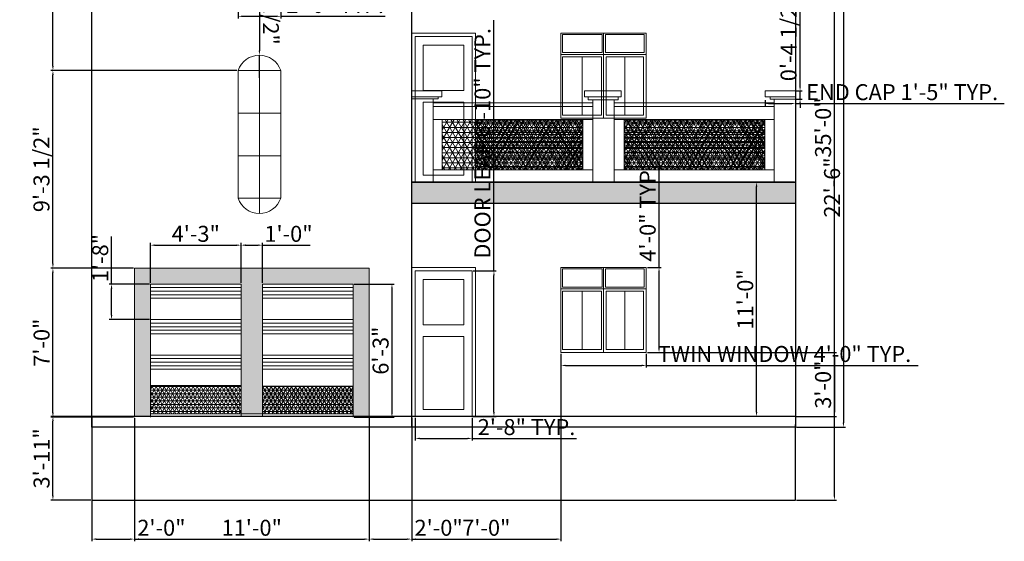
# Model space of a CAD drawing. Units: inches. Extents: x 107 to 1375, y 131 to 922.
# Tile 3 of 4: x 821 to 1375, y 327 to 621. Entities that reach past the tile are written whole.
import ezdxf

# ---------------------------------------------------------------- set-up
doc = ezdxf.new("R2010")
doc.units = ezdxf.units.IN
for name, color, linetype, lineweight in [('A-ANNO-DIMS', 2, 'Continuous', 13), ('A-DOOR-ELEV', 3, 'Continuous', 18), ('A-ELEV', 7, 'Continuous', 30), ('A-ELEV-RAIL', 7, 'Continuous', 18), ('A-GLAZ-ELEV', 4, 'Continuous', 18)]:
    doc.layers.add(name, color=color, linetype=linetype, lineweight=lineweight)
doc.layers.add('A-DOOR-PATT', color=18, linetype='Continuous', lineweight=13, true_color=0x000000)
doc.layers.add('A-ELEV-PATT', color=18, linetype='Continuous', lineweight=13, true_color=0x000000)
doc.styles.get("Standard").update_dxf_attribs({"font": 'arial.ttf'})
doc.dimstyles.new('ISO-25', dxfattribs={"dimtxt": 9, "dimasz": 2.5, "dimexe": 1.25, "dimexo": 0.625, "dimtad": 1, "dimlunit": 3, "dimtxsty": 'Standard', "dimcen": 2.5, "dimadec": 0, "dimazin": 0, "dimtfac": 1, "dimtmove": 0, "dimatfit": 3, "dimfxl": 1, "dimarcsym": 0})

# ---------------------------------------------------------------- blocks, each defined once
blk = doc.blocks.new('*D6')
at = {"layer": 'A-ANNO-DIMS', "color": 0, "lineweight": -2, "transparency": 16777216}
for p, q in [((1257.76, 661.18), (1285.35, 661.18)), ((1284.1, 658.68), (1284.1, 393.68)), ((1257.76, 391.18), (1285.35, 391.18))]:
    blk.add_line(p, q, dxfattribs=at)
at = {"layer": 'A-ANNO-DIMS', "color": 0, "transparency": 16777216}
for points in [[(1283.69, 658.68), (1284.52, 658.68), (1284.1, 661.18)], [(1283.69, 393.68), (1284.52, 393.68), (1284.1, 391.18)]]:
    blk.add_solid(points, dxfattribs=at)
at = {"layer": 'Defpoints', "color": 0, "transparency": 16777216}
for p in [(1257.14, 661.18), (1257.14, 391.18), (1284.1, 391.18)]:
    blk.add_point(p, dxfattribs=at)
at = {"layer": 'A-ANNO-DIMS', "color": 0, "transparency": 16777216, "insert": (1278.88, 526.18), "char_height": 9, "attachment_point": 5, "rotation": 90}
blk.add_mtext('22\'-6"', dxfattribs=at)
blk = doc.blocks.new('WINDOW-ELEV-TWIN-TRANSOM')
for p, q in [((0, 48), (0, 0)), ((0, 48), (48, 48)), ((24, 48), (24, 0)), ((48, 48), (48, 0)), ((0, 36), (48, 36)), ((11.87, 34.59), (11.87, 1.73)), ((36, 34.59), (36, 1.73)), ((48, 0), (0, 0))]:
    blk.add_line(p, q)
for points in [[(0.88, 47.17), (23.15, 47.17), (23.15, 36.96), (0.88, 36.96)], [(25.01, 47.17), (46.92, 47.17), (46.92, 36.96), (25.01, 36.96)], [(0.88, 34.59), (22.86, 34.59), (22.86, 1.73), (0.88, 1.73)], [(25.46, 34.59), (46.55, 34.59), (46.55, 1.73), (25.46, 1.73)]]:
    blk.add_lwpolyline(points, close=True)
blk = doc.blocks.new('WINDOW-ELEV-ROUND-END')
for p, q in [((12, 89.15), (12, 0)), ((0, 80.57), (0, 8.57)), ((24, 80.57), (0, 80.57)), ((24, 8.57), (24, 80.57)), ((24, 56.57), (0, 56.57)), ((24, 32.57), (0, 32.57)), ((24, 8.57), (0, 8.57))]:
    blk.add_line(p, q)
for centre, start, end in [((12, 76.46), 18.9145, 161.0855), ((12, 12.68), 198.9145, 341.0855)]:
    blk.add_arc(centre, 12.68, start, end)
blk = doc.blocks.new('DOOR-ELEV-TWO-PANEL-LEAF')
for p, q in [((0, 0), (0, 82)), ((0, 82), (32, 82)), ((32, 82), (32, 0))]:
    blk.add_line(p, q)
for points in [[(4.5, 77.24), (27.38, 77.24), (27.38, 51.66), (4.5, 51.66)], [(4.5, 45.15), (27.38, 45.15), (27.38, 3.9), (4.5, 3.9)]]:
    blk.add_lwpolyline(points, close=True)
blk = doc.blocks.new('GUARD-POST-LEFT')
for p, q in [((16.93, 51.4), (0, 51.4)), ((0, 51.4), (0, 48)), ((16.93, 48), (16.93, 51.4)), ((0, 48), (0, 0)), ((0, 48), (16.93, 48)), ((0, 46.97), (14.82, 46.97)), ((12, 46.97), (12, 0)), ((14.82, 46.97), (14.82, 48))]:
    blk.add_line(p, q)
blk = doc.blocks.new('GUARD-POST-CENTER')
for p, q in [((0, 51.4), (20.53, 51.4)), ((0, 51.4), (0, 48)), ((20.53, 48), (20.53, 51.4)), ((0, 48), (20.53, 48)), ((1.99, 48), (1.99, 46.37)), ((1.99, 46.37), (18.83, 46.37)), ((4.69, 0), (4.69, 46.37)), ((16.69, 0), (16.69, 46.37)), ((18.83, 46.37), (18.83, 48))]:
    blk.add_line(p, q)
blk = doc.blocks.new('GUARD-CAP-RIGHT')
for p, q in [((17.1, 4.57), (0, 4.57)), ((0, 4.57), (0, 1.16)), ((17.1, 1.16), (0, 1.16)), ((2.86, 1.16), (2.86, 0)), ((2.86, 0), (17.1, 0)), ((17.1, 1.16), (17.1, 4.57))]:
    blk.add_line(p, q)
blk = doc.blocks.new('*D34')
at = {"layer": 'A-ANNO-DIMS', "color": 0, "lineweight": -2, "transparency": 16777216}
for p, q in [((1125.14, 432.55), (1125.14, 424.73)), ((1173.14, 432.55), (1173.14, 424.73)), ((1127.64, 425.98), (1170.64, 425.98)), ((1173.14, 425.98), (1326.25, 425.98))]:
    blk.add_line(p, q, dxfattribs=at)
at = {"layer": 'A-ANNO-DIMS', "color": 0, "transparency": 16777216}
for points in [[(1127.64, 426.4), (1127.64, 425.56), (1125.14, 425.98)], [(1170.64, 426.4), (1170.64, 425.56), (1173.14, 425.98)]]:
    blk.add_solid(points, dxfattribs=at)
at = {"layer": 'Defpoints', "color": 0, "transparency": 16777216}
for p in [(1125.14, 433.18), (1173.14, 433.18), (1173.14, 425.98)]:
    blk.add_point(p, dxfattribs=at)
at = {"layer": 'A-ANNO-DIMS', "color": 0, "transparency": 16777216, "insert": (1250.94, 431.26), "char_height": 9, "attachment_point": 5}
blk.add_mtext('TWIN WINDOW 4\'-0" TYP.', dxfattribs=at)
blk = doc.blocks.new('*D35')
at = {"layer": 'A-ANNO-DIMS', "color": 0, "lineweight": -2, "transparency": 16777216}
for p, q in [((1180.34, 481.18), (1180.34, 540.15)), ((1173.76, 481.18), (1181.59, 481.18)), ((1180.34, 435.68), (1180.34, 478.68)), ((1173.76, 433.18), (1181.59, 433.18))]:
    blk.add_line(p, q, dxfattribs=at)
at = {"layer": 'A-ANNO-DIMS', "color": 0, "transparency": 16777216}
for points in [[(1179.92, 478.68), (1180.75, 478.68), (1180.34, 481.18)], [(1179.92, 435.68), (1180.75, 435.68), (1180.34, 433.18)]]:
    blk.add_solid(points, dxfattribs=at)
at = {"layer": 'Defpoints', "color": 0, "transparency": 16777216}
for p in [(1173.14, 481.18), (1180.34, 481.18), (1173.14, 433.18)]:
    blk.add_point(p, dxfattribs=at)
at = {"layer": 'A-ANNO-DIMS', "color": 0, "transparency": 16777216, "insert": (1175.12, 511.91), "char_height": 9, "attachment_point": 5, "rotation": 90}
blk.add_mtext('4\'-0" TYP.', dxfattribs=at)
blk = doc.blocks.new('*D37')
at = {"layer": 'A-ANNO-DIMS', "color": 0, "lineweight": -2, "transparency": 16777216}
for p, q in [((943.44, 635.37), (943.44, 621.37)), ((967.44, 635.37), (967.44, 621.37)), ((945.94, 622.62), (964.94, 622.62)), ((967.44, 622.62), (1026.2, 622.62))]:
    blk.add_line(p, q, dxfattribs=at)
at = {"layer": 'A-ANNO-DIMS', "color": 0, "transparency": 16777216}
for points in [[(945.94, 623.04), (945.94, 622.21), (943.44, 622.62)], [(964.94, 623.04), (964.94, 622.21), (967.44, 622.62)]]:
    blk.add_solid(points, dxfattribs=at)
at = {"layer": 'Defpoints', "color": 0, "transparency": 16777216}
for p in [(943.44, 636), (967.44, 636), (967.44, 622.62)]:
    blk.add_point(p, dxfattribs=at)
at = {"layer": 'A-ANNO-DIMS', "color": 0, "transparency": 16777216, "insert": (998.07, 627.84), "char_height": 9, "attachment_point": 5}
blk.add_mtext('2\'-0" TYP.', dxfattribs=at)
blk = doc.blocks.new('*D38')
at = {"layer": 'A-ANNO-DIMS', "color": 0, "lineweight": -2, "transparency": 16777216}
for p, q in [((1087.44, 479.18), (1087.44, 620.48)), ((1075.76, 479.18), (1088.69, 479.18)), ((1087.44, 399.68), (1087.44, 476.68)), ((1075.76, 397.18), (1088.69, 397.18))]:
    blk.add_line(p, q, dxfattribs=at)
at = {"layer": 'A-ANNO-DIMS', "color": 0, "transparency": 16777216}
for points in [[(1087.02, 476.68), (1087.85, 476.68), (1087.44, 479.18)], [(1087.02, 399.68), (1087.85, 399.68), (1087.44, 397.18)]]:
    blk.add_solid(points, dxfattribs=at)
at = {"layer": 'Defpoints', "color": 0, "transparency": 16777216}
for p in [(1075.14, 479.18), (1087.44, 479.18), (1075.14, 397.18)]:
    blk.add_point(p, dxfattribs=at)
at = {"layer": 'A-ANNO-DIMS', "color": 0, "transparency": 16777216, "insert": (1082.15, 551.08), "char_height": 9, "attachment_point": 5, "rotation": 90}
blk.add_mtext('DOOR LEAF 6\'-10" TYP.', dxfattribs=at)
blk = doc.blocks.new('*D39')
at = {"layer": 'A-ANNO-DIMS', "color": 0, "lineweight": -2, "transparency": 16777216}
for p, q in [((1043.14, 396.55), (1043.14, 383.63)), ((1075.14, 396.55), (1075.14, 383.63)), ((1045.64, 384.88), (1072.64, 384.88)), ((1075.14, 384.88), (1133.9, 384.88))]:
    blk.add_line(p, q, dxfattribs=at)
at = {"layer": 'A-ANNO-DIMS', "color": 0, "transparency": 16777216}
for points in [[(1045.64, 385.3), (1045.64, 384.46), (1043.14, 384.88)], [(1072.64, 385.3), (1072.64, 384.46), (1075.14, 384.88)]]:
    blk.add_solid(points, dxfattribs=at)
at = {"layer": 'Defpoints', "color": 0, "transparency": 16777216}
for p in [(1043.14, 397.18), (1075.14, 397.18), (1075.14, 384.88)]:
    blk.add_point(p, dxfattribs=at)
at = {"layer": 'A-ANNO-DIMS', "color": 0, "transparency": 16777216, "insert": (1105.77, 390.1), "char_height": 9, "attachment_point": 5}
blk.add_mtext('2\'-8" TYP.', dxfattribs=at)
blk = doc.blocks.new('*D44')
at = {"layer": 'A-ANNO-DIMS', "color": 0, "lineweight": -2, "transparency": 16777216}
for p, q in [((1240.04, 575.39), (1240.04, 572.2)), ((1242.54, 573.45), (1254.64, 573.45)), ((1257.14, 575.39), (1257.14, 572.2)), ((1257.14, 573.45), (1374.66, 573.45))]:
    blk.add_line(p, q, dxfattribs=at)
at = {"layer": 'A-ANNO-DIMS', "color": 0, "transparency": 16777216}
for points in [[(1242.54, 573.87), (1242.54, 573.03), (1240.04, 573.45)], [(1254.64, 573.87), (1254.64, 573.03), (1257.14, 573.45)]]:
    blk.add_solid(points, dxfattribs=at)
at = {"layer": 'Defpoints', "color": 0, "transparency": 16777216}
for p in [(1240.04, 576.02), (1257.14, 576.02), (1257.14, 573.45)]:
    blk.add_point(p, dxfattribs=at)
at = {"layer": 'A-ANNO-DIMS', "color": 0, "transparency": 16777216, "insert": (1317.15, 578.73), "char_height": 9, "attachment_point": 5}
blk.add_mtext('END CAP 1\'-5" TYP.', dxfattribs=at)
blk = doc.blocks.new('*D45')
at = {"layer": 'A-ANNO-DIMS', "color": 0, "lineweight": -2, "transparency": 16777216}
for p, q in [((1259.7, 583.08), (1259.7, 662.66)), ((1257.76, 580.58), (1260.95, 580.58)), ((1259.7, 576.02), (1259.7, 580.58)), ((1257.76, 576.02), (1260.95, 576.02)), ((1259.7, 573.52), (1259.7, 571.02))]:
    blk.add_line(p, q, dxfattribs=at)
at = {"layer": 'A-ANNO-DIMS', "color": 0, "transparency": 16777216}
for points in [[(1259.28, 583.08), (1260.12, 583.08), (1259.7, 580.58)], [(1259.28, 573.52), (1260.12, 573.52), (1259.7, 576.02)]]:
    blk.add_solid(points, dxfattribs=at)
at = {"layer": 'Defpoints', "color": 0, "transparency": 16777216}
for p in [(1257.14, 580.58), (1259.7, 580.58), (1257.14, 576.02)]:
    blk.add_point(p, dxfattribs=at)
at = {"layer": 'A-ANNO-DIMS', "color": 0, "transparency": 16777216, "insert": (1254.42, 624.12), "char_height": 9, "attachment_point": 5, "rotation": 90}
blk.add_mtext('0\'-4 1/2" TYP.', dxfattribs=at)
blk = doc.blocks.new('*D58')
at = {"layer": 'A-ANNO-DIMS', "color": 0, "lineweight": -2, "transparency": 16777216}
for p, q in [((1071.8, 769.86), (1280.29, 769.86)), ((1279.04, 352.56), (1279.04, 767.36)), ((1257.76, 350.06), (1280.29, 350.06))]:
    blk.add_line(p, q, dxfattribs=at)
at = {"layer": 'A-ANNO-DIMS', "color": 0, "transparency": 16777216}
for points in [[(1278.62, 767.36), (1279.45, 767.36), (1279.04, 769.86)], [(1278.62, 352.56), (1279.45, 352.56), (1279.04, 350.06)]]:
    blk.add_solid(points, dxfattribs=at)
at = {"layer": 'Defpoints', "color": 0, "transparency": 16777216}
for p in [(1071.17, 769.86), (1279.04, 769.86), (1257.14, 350.06)]:
    blk.add_point(p, dxfattribs=at)
at = {"layer": 'A-ANNO-DIMS', "color": 0, "transparency": 16777216, "insert": (1273.81, 559.96), "char_height": 9, "attachment_point": 5, "rotation": 90}
blk.add_mtext('35\'-0"', dxfattribs=at)
blk = doc.blocks.new('*D59')
at = {"layer": 'A-ANNO-DIMS', "color": 0, "lineweight": -2, "transparency": 16777216}
for p, q in [((861.14, 396.55), (861.14, 326.91)), ((885.13, 396.19), (885.13, 326.91)), ((863.64, 328.16), (882.63, 328.16)), ((885.13, 328.16), (912.96, 328.16))]:
    blk.add_line(p, q, dxfattribs=at)
at = {"layer": 'A-ANNO-DIMS', "color": 0, "transparency": 16777216}
for points in [[(863.64, 328.58), (863.64, 327.75), (861.14, 328.16)], [(882.63, 328.58), (882.63, 327.75), (885.13, 328.16)]]:
    blk.add_solid(points, dxfattribs=at)
at = {"layer": 'Defpoints', "color": 0, "transparency": 16777216}
for p in [(861.14, 397.18), (885.13, 396.81), (885.13, 328.16)]:
    blk.add_point(p, dxfattribs=at)
at = {"layer": 'A-ANNO-DIMS', "color": 0, "transparency": 16777216, "insert": (900.3, 333.38), "char_height": 9, "attachment_point": 5}
blk.add_mtext('2\'-0"', dxfattribs=at)
blk = doc.blocks.new('*D60')
at = {"layer": 'A-ANNO-DIMS', "color": 0, "lineweight": -2, "transparency": 16777216}
for p, q in [((885.13, 396.19), (885.13, 326.91)), ((1017.13, 396.19), (1017.13, 326.91)), ((887.63, 328.16), (1014.63, 328.16))]:
    blk.add_line(p, q, dxfattribs=at)
at = {"layer": 'A-ANNO-DIMS', "color": 0, "transparency": 16777216}
for points in [[(887.63, 328.58), (887.63, 327.75), (885.13, 328.16)], [(1014.63, 328.58), (1014.63, 327.75), (1017.13, 328.16)]]:
    blk.add_solid(points, dxfattribs=at)
at = {"layer": 'Defpoints', "color": 0, "transparency": 16777216}
for p in [(885.13, 396.81), (1017.13, 396.81), (1017.13, 328.16)]:
    blk.add_point(p, dxfattribs=at)
at = {"layer": 'A-ANNO-DIMS', "color": 0, "transparency": 16777216, "insert": (951.13, 333.38), "char_height": 9, "attachment_point": 5}
blk.add_mtext('11\'-0"', dxfattribs=at)
blk = doc.blocks.new('*D61')
at = {"layer": 'A-ANNO-DIMS', "color": 0, "lineweight": -2, "transparency": 16777216}
for p, q in [((1017.13, 396.19), (1017.13, 326.91)), ((1041.14, 396.55), (1041.14, 326.91)), ((1019.63, 328.16), (1038.64, 328.16)), ((1041.14, 328.16), (1068.96, 328.16))]:
    blk.add_line(p, q, dxfattribs=at)
at = {"layer": 'A-ANNO-DIMS', "color": 0, "transparency": 16777216}
for points in [[(1019.63, 328.58), (1019.63, 327.75), (1017.13, 328.16)], [(1038.64, 328.58), (1038.64, 327.75), (1041.14, 328.16)]]:
    blk.add_solid(points, dxfattribs=at)
at = {"layer": 'Defpoints', "color": 0, "transparency": 16777216}
for p in [(1017.13, 396.81), (1041.14, 397.18), (1041.14, 328.16)]:
    blk.add_point(p, dxfattribs=at)
at = {"layer": 'A-ANNO-DIMS', "color": 0, "transparency": 16777216, "insert": (1056.3, 333.38), "char_height": 9, "attachment_point": 5}
blk.add_mtext('2\'-0"', dxfattribs=at)
blk = doc.blocks.new('*D62')
at = {"layer": 'A-ANNO-DIMS', "color": 0, "lineweight": -2, "transparency": 16777216}
for p, q in [((1125.14, 432.55), (1125.14, 326.91)), ((1041.14, 396.55), (1041.14, 326.91)), ((1043.64, 328.16), (1122.64, 328.16))]:
    blk.add_line(p, q, dxfattribs=at)
at = {"layer": 'A-ANNO-DIMS', "color": 0, "transparency": 16777216}
for points in [[(1043.64, 328.58), (1043.64, 327.75), (1041.14, 328.16)], [(1122.64, 328.58), (1122.64, 327.75), (1125.14, 328.16)]]:
    blk.add_solid(points, dxfattribs=at)
at = {"layer": 'Defpoints', "color": 0, "transparency": 16777216}
for p in [(1125.14, 433.18), (1041.14, 397.18), (1125.14, 328.16)]:
    blk.add_point(p, dxfattribs=at)
at = {"layer": 'A-ANNO-DIMS', "color": 0, "transparency": 16777216, "insert": (1083.14, 333.38), "char_height": 9, "attachment_point": 5}
blk.add_mtext('7\'-0"', dxfattribs=at)
blk = doc.blocks.new('*D63')
at = {"layer": 'A-ANNO-DIMS', "color": 0, "lineweight": -2, "transparency": 16777216}
for p, q in [((860.51, 397.18), (837.99, 397.18)), ((839.24, 352.56), (839.24, 394.68)), ((860.51, 350.06), (837.99, 350.06))]:
    blk.add_line(p, q, dxfattribs=at)
at = {"layer": 'A-ANNO-DIMS', "color": 0, "transparency": 16777216}
for points in [[(838.82, 394.68), (839.65, 394.68), (839.24, 397.18)], [(838.82, 352.56), (839.65, 352.56), (839.24, 350.06)]]:
    blk.add_solid(points, dxfattribs=at)
at = {"layer": 'Defpoints', "color": 0, "transparency": 16777216}
for p in [(839.24, 397.18), (861.14, 397.18), (861.14, 350.06)]:
    blk.add_point(p, dxfattribs=at)
at = {"layer": 'A-ANNO-DIMS', "color": 0, "transparency": 16777216, "insert": (834.01, 373.62), "char_height": 9, "attachment_point": 5, "rotation": 90}
blk.add_mtext('3\'-11"', dxfattribs=at)
blk = doc.blocks.new('*D64')
at = {"layer": 'A-ANNO-DIMS', "color": 0, "lineweight": -2, "transparency": 16777216}
for p, q in [((884.51, 480.81), (837.99, 480.81)), ((839.24, 399.31), (839.24, 478.31)), ((884.51, 396.81), (837.99, 396.81))]:
    blk.add_line(p, q, dxfattribs=at)
at = {"layer": 'A-ANNO-DIMS', "color": 0, "transparency": 16777216}
for points in [[(838.82, 478.31), (839.65, 478.31), (839.24, 480.81)], [(838.82, 399.31), (839.65, 399.31), (839.24, 396.81)]]:
    blk.add_solid(points, dxfattribs=at)
at = {"layer": 'Defpoints', "color": 0, "transparency": 16777216}
for p in [(839.24, 480.81), (885.13, 480.81), (885.13, 396.81)]:
    blk.add_point(p, dxfattribs=at)
at = {"layer": 'A-ANNO-DIMS', "color": 0, "transparency": 16777216, "insert": (834.02, 438.81), "char_height": 9, "attachment_point": 5, "rotation": 90}
blk.add_mtext('7\'-0"', dxfattribs=at)
blk = doc.blocks.new('*D65')
at = {"layer": 'A-ANNO-DIMS', "color": 0, "lineweight": -2, "transparency": 16777216}
for p, q in [((942.82, 592.12), (837.99, 592.12)), ((839.24, 483.31), (839.24, 589.62)), ((884.51, 480.81), (837.99, 480.81))]:
    blk.add_line(p, q, dxfattribs=at)
at = {"layer": 'A-ANNO-DIMS', "color": 0, "transparency": 16777216}
for points in [[(838.82, 589.62), (839.65, 589.62), (839.24, 592.12)], [(838.82, 483.31), (839.65, 483.31), (839.24, 480.81)]]:
    blk.add_solid(points, dxfattribs=at)
at = {"layer": 'Defpoints', "color": 0, "transparency": 16777216}
for p in [(839.24, 592.12), (943.44, 592.12), (885.13, 480.81)]:
    blk.add_point(p, dxfattribs=at)
at = {"layer": 'A-ANNO-DIMS', "color": 0, "transparency": 16777216, "insert": (833.95, 536.47), "char_height": 9, "attachment_point": 5, "rotation": 90}
blk.add_mtext('9\'-3 1/2"', dxfattribs=at)
blk = doc.blocks.new('*D66')
at = {"layer": 'A-ANNO-DIMS', "color": 0, "lineweight": -2, "transparency": 16777216}
for p, q in [((942.82, 716.57), (837.99, 716.57)), ((839.24, 594.62), (839.24, 714.07)), ((942.82, 592.12), (837.99, 592.12))]:
    blk.add_line(p, q, dxfattribs=at)
at = {"layer": 'A-ANNO-DIMS', "color": 0, "transparency": 16777216}
for points in [[(838.82, 714.07), (839.65, 714.07), (839.24, 716.57)], [(838.82, 594.62), (839.65, 594.62), (839.24, 592.12)]]:
    blk.add_solid(points, dxfattribs=at)
at = {"layer": 'Defpoints', "color": 0, "transparency": 16777216}
for p in [(839.24, 716.57), (943.44, 716.57), (943.44, 592.12)]:
    blk.add_point(p, dxfattribs=at)
at = {"layer": 'A-ANNO-DIMS', "color": 0, "transparency": 16777216, "insert": (833.96, 654.34), "char_height": 9, "attachment_point": 5, "rotation": 90}
blk.add_mtext('10\'-4 1/2"', dxfattribs=at)
blk = doc.blocks.new('*D67')
at = {"layer": 'A-ANNO-DIMS', "color": 0, "lineweight": -2, "transparency": 16777216}
for p, q in [((1256.51, 529.18), (1233.99, 529.18)), ((1235.24, 399.68), (1235.24, 526.68)), ((1256.51, 397.18), (1233.99, 397.18))]:
    blk.add_line(p, q, dxfattribs=at)
at = {"layer": 'A-ANNO-DIMS', "color": 0, "transparency": 16777216}
for points in [[(1234.82, 526.68), (1235.65, 526.68), (1235.24, 529.18)], [(1234.82, 399.68), (1235.65, 399.68), (1235.24, 397.18)]]:
    blk.add_solid(points, dxfattribs=at)
at = {"layer": 'Defpoints', "color": 0, "transparency": 16777216}
for p in [(1235.24, 529.18), (1257.14, 529.18), (1257.14, 397.18)]:
    blk.add_point(p, dxfattribs=at)
at = {"layer": 'A-ANNO-DIMS', "color": 0, "transparency": 16777216, "insert": (1230.02, 463.18), "char_height": 9, "attachment_point": 5, "rotation": 90}
blk.add_mtext('11\'-0"', dxfattribs=at)
blk = doc.blocks.new('*D68')
at = {"layer": 'A-ANNO-DIMS', "color": 0, "lineweight": -2, "transparency": 16777216}
for p, q in [((1173.76, 433.18), (1280.29, 433.18)), ((1279.04, 430.68), (1279.04, 399.68)), ((1257.76, 397.18), (1280.29, 397.18))]:
    blk.add_line(p, q, dxfattribs=at)
at = {"layer": 'A-ANNO-DIMS', "color": 0, "transparency": 16777216}
for points in [[(1278.62, 430.68), (1279.45, 430.68), (1279.04, 433.18)], [(1278.62, 399.68), (1279.45, 399.68), (1279.04, 397.18)]]:
    blk.add_solid(points, dxfattribs=at)
at = {"layer": 'Defpoints', "color": 0, "transparency": 16777216}
for p in [(1173.14, 433.18), (1257.14, 397.18), (1279.04, 397.18)]:
    blk.add_point(p, dxfattribs=at)
at = {"layer": 'A-ANNO-DIMS', "color": 0, "transparency": 16777216, "insert": (1273.81, 415.18), "char_height": 9, "attachment_point": 5, "rotation": 90}
blk.add_mtext('3\'-0"', dxfattribs=at)
blk = doc.blocks.new('*D72')
at = {"layer": 'A-ANNO-DIMS', "color": 0, "lineweight": -2, "transparency": 16777216}
for p, q in [((894.13, 472.44), (894.13, 494.96)), ((896.63, 493.71), (942.63, 493.71)), ((945.13, 472.44), (945.13, 494.96))]:
    blk.add_line(p, q, dxfattribs=at)
at = {"layer": 'A-ANNO-DIMS', "color": 0, "transparency": 16777216}
for points in [[(896.63, 494.13), (896.63, 493.3), (894.13, 493.71)], [(942.63, 494.13), (942.63, 493.3), (945.13, 493.71)]]:
    blk.add_solid(points, dxfattribs=at)
at = {"layer": 'Defpoints', "color": 0, "transparency": 16777216}
for p in [(945.13, 493.71), (894.13, 471.81), (945.13, 471.81)]:
    blk.add_point(p, dxfattribs=at)
at = {"layer": 'A-ANNO-DIMS', "color": 0, "transparency": 16777216, "insert": (919.63, 498.94), "char_height": 9, "attachment_point": 5}
blk.add_mtext('4\'-3"', dxfattribs=at)
blk = doc.blocks.new('*D73')
at = {"layer": 'A-ANNO-DIMS', "color": 0, "lineweight": -2, "transparency": 16777216}
for p, q in [((945.13, 472.44), (945.13, 494.96)), ((947.63, 493.71), (954.63, 493.71)), ((957.13, 472.44), (957.13, 494.96)), ((957.13, 493.71), (983.96, 493.71))]:
    blk.add_line(p, q, dxfattribs=at)
at = {"layer": 'A-ANNO-DIMS', "color": 0, "transparency": 16777216}
for points in [[(947.63, 494.13), (947.63, 493.3), (945.13, 493.71)], [(954.63, 494.13), (954.63, 493.3), (957.13, 493.71)]]:
    blk.add_solid(points, dxfattribs=at)
at = {"layer": 'Defpoints', "color": 0, "transparency": 16777216}
for p in [(957.13, 493.71), (945.13, 471.81), (957.13, 471.81)]:
    blk.add_point(p, dxfattribs=at)
at = {"layer": 'A-ANNO-DIMS', "color": 0, "transparency": 16777216, "insert": (971.8, 498.93), "char_height": 9, "attachment_point": 5}
blk.add_mtext('1\'-0"', dxfattribs=at)
blk = doc.blocks.new('*D77')
at = {"layer": 'A-ANNO-DIMS', "color": 0, "lineweight": -2, "transparency": 16777216}
for p, q in [((872.23, 471.81), (872.23, 498.64)), ((893.51, 471.81), (870.98, 471.81)), ((872.23, 454.31), (872.23, 469.31)), ((893.51, 451.81), (870.98, 451.81))]:
    blk.add_line(p, q, dxfattribs=at)
at = {"layer": 'A-ANNO-DIMS', "color": 0, "transparency": 16777216}
for points in [[(871.82, 469.31), (872.65, 469.31), (872.23, 471.81)], [(871.82, 454.31), (872.65, 454.31), (872.23, 451.81)]]:
    blk.add_solid(points, dxfattribs=at)
at = {"layer": 'Defpoints', "color": 0, "transparency": 16777216}
for p in [(872.23, 471.81), (894.13, 471.81), (894.13, 451.81)]:
    blk.add_point(p, dxfattribs=at)
at = {"layer": 'A-ANNO-DIMS', "color": 0, "transparency": 16777216, "insert": (867.01, 486.48), "char_height": 9, "attachment_point": 5, "rotation": 90}
blk.add_mtext('1\'-8"', dxfattribs=at)
blk = doc.blocks.new('*D78')
at = {"layer": 'A-ANNO-DIMS', "color": 0, "lineweight": -2, "transparency": 16777216}
for p, q in [((1008.76, 471.81), (1031.28, 471.81)), ((1030.03, 469.31), (1030.03, 399.31)), ((1008.76, 396.81), (1031.28, 396.81))]:
    blk.add_line(p, q, dxfattribs=at)
at = {"layer": 'A-ANNO-DIMS', "color": 0, "transparency": 16777216}
for points in [[(1029.62, 469.31), (1030.45, 469.31), (1030.03, 471.81)], [(1029.62, 399.31), (1030.45, 399.31), (1030.03, 396.81)]]:
    blk.add_solid(points, dxfattribs=at)
at = {"layer": 'Defpoints', "color": 0, "transparency": 16777216}
for p in [(1008.13, 471.81), (1008.13, 396.81), (1030.03, 396.81)]:
    blk.add_point(p, dxfattribs=at)
at = {"layer": 'A-ANNO-DIMS', "color": 0, "transparency": 16777216, "insert": (1024.81, 434.31), "char_height": 9, "attachment_point": 5, "rotation": 90}
blk.add_mtext('6\'-3"', dxfattribs=at)
blk = doc.blocks.new('*D81')
at = {"layer": 'A-ANNO-DIMS', "color": 0, "lineweight": -2, "transparency": 16777216}
for p, q in [((955.44, 680.15), (955.44, 603.19)), ((955.44, 588.01), (955.44, 600.69))]:
    blk.add_line(p, q, dxfattribs=at)
at = {"layer": 'A-ANNO-DIMS', "color": 0, "transparency": 16777216}
blk.add_solid([(955.86, 603.19), (955.02, 603.19), (955.44, 600.69)], dxfattribs=at)
at = {"layer": 'Defpoints', "color": 0, "transparency": 16777216}
for p in [(955.44, 600.69), (955.44, 588.01)]:
    blk.add_point(p, dxfattribs=at)
at = {"layer": 'A-ANNO-DIMS', "color": 0, "transparency": 16777216, "insert": (960.72, 642.92), "char_height": 9, "attachment_point": 5, "rotation": 270.0018}
blk.add_mtext('4X R1\'-0 1/2"', dxfattribs=at)

msp = doc.modelspace()

# ---------------------------------------------------------------- hatches: boundary and pattern name
at = {"layer": 'A-DOOR-PATT'}
h = msp.add_hatch(color=256, dxfattribs=at)
h.dxf.hatch_style = 1
h.paths.add_polyline_path([(1017.133, 480.813), (885.133, 480.813), (885.133, 397.179), (894.133, 397.179), (894.133, 471.813), (945.133, 471.813), (945.133, 398.813), (957.133, 398.813), (957.133, 471.813), (1008.133, 471.813), (1008.133, 447.813), (1017.133, 447.813)])
h = msp.add_hatch(color=256, dxfattribs=at)
h.dxf.hatch_style = 1
h.paths.add_polyline_path([(1017.133, 480.813), (885.133, 480.813), (885.133, 397.179), (894.133, 397.179), (894.133, 471.813), (945.133, 471.813), (945.133, 398.813), (957.133, 398.813), (957.133, 471.813), (1008.133, 471.813), (1008.133, 397.179), (1017.133, 397.179)])
at = {"layer": 'A-ELEV-PATT'}
h = msp.add_hatch(color=256, dxfattribs=at)
h.dxf.hatch_style = 1
h.paths.add_polyline_path([(1257.136, 661.179), (1041.136, 661.179), (1041.136, 649.179), (1257.136, 649.179)])
h.paths.add_polyline_path([(1257.136, 529.179), (1041.136, 529.179), (1041.136, 517.179), (1257.136, 517.179)])
h = msp.add_hatch(dxfattribs=at)
h.set_pattern_fill('NET3', color=256, scale=0.63)
h.paths.add_polyline_path([(945.133, 414.712), (894.133, 414.712), (894.133, 398.813), (945.133, 398.813)])
h.paths.add_polyline_path([(1008.133, 414.387), (957.133, 414.387), (957.133, 398.813), (1008.133, 398.813)])
h.paths.add_polyline_path([(1239.797, 564.403), (1160.646, 564.403), (1160.646, 536.106), (1239.797, 536.106)])
h.paths.add_polyline_path([(1137.409, 564.403), (1077.136, 564.403), (1077.136, 536.106), (1137.409, 536.106)])
h = msp.add_hatch(dxfattribs=at)
h.set_pattern_fill('NET3', color=256, scale=0.9)
h.paths.add_polyline_path([(1137.409, 564.403), (1058.258, 564.403), (1058.258, 536.106), (1137.409, 536.106)])
h.paths.add_polyline_path([(1239.797, 564.403), (1160.646, 564.403), (1160.646, 536.106), (1239.797, 536.106)])

# ---------------------------------------------------------------- linework, layer by layer
at = {"layer": 'A-DOOR-ELEV'}
for p, q in [((1041.136, 529.179), (1041.136, 613.179)), ((1041.136, 613.179), (1077.136, 613.179)), ((1077.136, 613.179), (1077.136, 529.179)), ((1041.136, 529.179), (1077.136, 529.179)), ((885.133, 396.813), (885.133, 480.813)), ((885.133, 480.813), (1017.133, 480.813)), ((1017.133, 480.813), (1017.133, 396.813)), ((1041.136, 397.179), (1041.136, 481.179)), ((1041.136, 481.179), (1077.136, 481.179)), ((1077.136, 481.179), (1077.136, 397.179)), ((894.133, 471.813), (945.133, 471.813)), ((894.133, 396.813), (894.133, 471.813)), ((945.133, 471.813), (945.133, 397.179)), ((957.133, 471.813), (957.133, 397.179)), ((957.133, 471.813), (1008.133, 471.813)), ((1008.133, 471.813), (1008.133, 396.813)), ((894.133, 469.813), (945.133, 469.813)), ((894.133, 467.813), (945.133, 467.813)), ((894.133, 465.813), (945.133, 465.813)), ((957.133, 469.813), (1008.133, 469.813)), ((957.133, 467.813), (1008.133, 467.813)), ((957.133, 465.813), (1008.133, 465.813)), ((894.133, 463.813), (945.133, 463.813)), ((957.133, 463.813), (1008.133, 463.813)), ((894.133, 451.813), (945.133, 451.813)), ((894.133, 449.813), (945.133, 449.813)), ((957.133, 451.813), (1008.133, 451.813)), ((957.133, 449.813), (1008.133, 449.813)), ((894.133, 447.813), (945.133, 447.813)), ((894.133, 445.813), (945.133, 445.813)), ((894.133, 443.813), (945.133, 443.813)), ((957.133, 447.813), (1008.133, 447.813)), ((957.133, 445.813), (1008.133, 445.813)), ((957.133, 443.813), (1008.133, 443.813)), ((894.133, 431.813), (945.133, 431.813)), ((894.133, 429.813), (945.133, 429.813)), ((894.133, 427.813), (945.133, 427.813)), ((957.133, 431.813), (1008.133, 431.813)), ((957.133, 429.813), (1008.133, 429.813)), ((957.133, 427.813), (1008.133, 427.813)), ((894.133, 425.813), (945.133, 425.813)), ((894.133, 423.813), (945.133, 423.813)), ((957.133, 425.813), (1008.133, 425.813)), ((957.133, 423.813), (1008.133, 423.813)), ((894.133, 414.712), (945.133, 414.712)), ((957.133, 414.387), (1008.133, 414.387)), ((885.133, 396.813), (885.133, 398.813)), ((894.133, 398.813), (1008.133, 398.813))]:
    msp.add_line(p, q, dxfattribs=at)
at = {"layer": 'A-ELEV'}
for p, q in [((861.136, 391.179), (861.136, 751.179)), ((1041.136, 391.179), (1041.136, 751.179)), ((1257.136, 673.43), (1257.136, 394.43)), ((1250.832, 529.179), (1041.136, 529.179)), ((1041.136, 529.179), (1257.136, 529.179)), ((1257.136, 517.179), (1041.136, 517.179)), ((1257.136, 397.179), (861.136, 397.179)), ((1257.136, 394.43), (1257.136, 391.179)), ((1242.832, 391.179), (861.136, 391.179)), ((861.136, 391.179), (861.136, 350.065)), ((1257.136, 391.179), (1242.832, 391.179)), ((1257.136, 350.065), (1257.136, 392.805)), ((861.136, 350.065), (1257.136, 350.065))]:
    msp.add_line(p, q, dxfattribs=at)
at = {"layer": 'A-ELEV-RAIL'}
for p, q in [((1257.136, 529.179), (1257.136, 577.179)), ((1053.136, 573.817), (1143.136, 573.817)), ((1053.136, 571.817), (1143.136, 571.817)), ((1155.136, 573.817), (1245.136, 573.817)), ((1155.136, 571.817), (1245.136, 571.817)), ((1245.136, 529.179), (1245.136, 576.015)), ((1053.136, 564.403), (1058.258, 564.403)), ((1137.409, 564.403), (1143.136, 564.403)), ((1160.646, 564.403), (1155.136, 564.403)), ((1239.797, 564.403), (1245.136, 564.403)), ((1058.258, 536.106), (1053.136, 536.106)), ((1137.409, 536.106), (1143.136, 536.106)), ((1160.646, 536.106), (1155.136, 536.106)), ((1239.797, 536.106), (1245.136, 536.106))]:
    msp.add_line(p, q, dxfattribs=at)
for points in [[(1058.258, 564.403), (1137.409, 564.403), (1137.409, 536.106), (1058.258, 536.106)], [(1160.646, 564.403), (1239.797, 564.403), (1239.797, 536.106), (1160.646, 536.106)]]:
    msp.add_lwpolyline(points, close=True, dxfattribs=at)

# ---------------------------------------------------------------- block references
at = {"layer": 'A-DOOR-ELEV'}
for p in [(1043.136, 529.179), (1043.136, 397.179)]:
    msp.add_blockref('DOOR-ELEV-TWO-PANEL-LEAF', p, dxfattribs=at)
at = {"layer": 'A-ELEV-RAIL'}
for name, p in [('GUARD-POST-LEFT', (1041.136, 529.179)), ('GUARD-POST-CENTER', (1138.451, 529.179)), ('GUARD-CAP-RIGHT', (1240.04, 576.015))]:
    msp.add_blockref(name, p, dxfattribs=at)
at = {"layer": 'A-GLAZ-ELEV'}
for name, p in [('WINDOW-ELEV-TWIN-TRANSOM', (1125.136, 565.179)), ('WINDOW-ELEV-ROUND-END', (943.44, 511.544)), ('WINDOW-ELEV-TWIN-TRANSOM', (1125.136, 433.179))]:
    msp.add_blockref(name, p, dxfattribs=at)

# ---------------------------------------------------------------- dimensions: what is measured, and where the dimension line sits
at = {"layer": 'A-ANNO-DIMS'}
for base, p1, p2, angle, override, picture, middle in [((1279.036, 769.862), (1257.136, 350.065), (1071.173, 769.862), 90, {"dimdec": 1, "dimlfac": 1, "dimrnd": 0, "dimzin": 1, "dimdsep": 46, "dimlunit": 4, "dimfrac": 2}, '*D58', (1273.813, 559.963)), ((839.236, 716.57), (943.44, 592.118), (943.44, 716.57), 90, {"dimdec": 1, "dimlfac": 1, "dimrnd": 0, "dimzin": 1, "dimdsep": 46, "dimlunit": 4, "dimfrac": 2}, '*D66', (833.958, 654.344)), ((1284.102, 391.179), (1257.136, 661.179), (1257.136, 391.179), 90, {"dimclrd": 0, "dimclre": 0, "dimclrt": 0}, '*D6', (1278.882, 526.179)), ((839.236, 592.118), (885.133, 480.813), (943.44, 592.118), 90, {"dimdec": 1, "dimlfac": 1, "dimrnd": 0, "dimzin": 1, "dimdsep": 46, "dimlunit": 4, "dimfrac": 2}, '*D65', (833.955, 536.465)), ((1235.236, 529.179), (1257.136, 397.179), (1257.136, 529.179), 90, {"dimdec": 1, "dimlfac": 1, "dimrnd": 0, "dimzin": 1, "dimdsep": 46, "dimlunit": 4, "dimfrac": 2}, '*D67', (1230.016, 463.179)), ((872.233, 471.813), (894.133, 451.813), (894.133, 471.813), 90, {"dimdec": 1, "dimlfac": 1, "dimrnd": 0, "dimzin": 1, "dimdsep": 46, "dimlunit": 4, "dimfrac": 2}, '*D77', (867.013, 486.477)), ((839.236, 480.813), (885.133, 396.813), (885.133, 480.813), 90, {"dimdec": 1, "dimlfac": 1, "dimrnd": 0, "dimzin": 1, "dimdsep": 46, "dimlunit": 4, "dimfrac": 2}, '*D64', (834.016, 438.813)), ((1030.033, 396.813), (1008.133, 471.813), (1008.133, 396.813), 270, {"dimdec": 1, "dimlfac": 1, "dimrnd": 0, "dimzin": 1, "dimdsep": 46, "dimlunit": 4, "dimfrac": 2}, '*D78', (1024.81, 434.313)), ((1279.036, 397.179), (1173.136, 433.179), (1257.136, 397.179), 90, {"dimdec": 1, "dimlfac": 1, "dimrnd": 0, "dimzin": 1, "dimdsep": 46, "dimlunit": 4, "dimfrac": 2}, '*D68', (1273.813, 415.179)), ((839.236, 397.179), (861.136, 350.065), (861.136, 397.179), 90, {"dimdec": 1, "dimlfac": 1, "dimrnd": 0, "dimzin": 1, "dimdsep": 46, "dimlunit": 4, "dimfrac": 2}, '*D63', (834.013, 373.622))]:
    dim = msp.add_linear_dim(base=base, p1=p1, p2=p2, angle=angle, dimstyle='ISO-25', override=override, dxfattribs=at)
    dim.commit()
    dim.dimension.update_dxf_attribs({"geometry": picture, "text_midpoint": middle})
dim = msp.add_radius_dim(center=(955.44, 588.006), mpoint=(955.44, 600.691), text='4X <>', dimstyle='ISO-25', override={"dimdec": 1, "dimlfac": 1, "dimrnd": 0, "dimzin": 1, "dimdsep": 46, "dimlunit": 4, "dimfrac": 2}, dxfattribs=at)
dim.commit()
dim.dimension.update_dxf_attribs({"geometry": '*D81', "text_midpoint": (960.717, 642.92)})
for base, p1, p2, text, picture, middle in [((1259.701, 580.583), (1257.136, 576.015), (1257.136, 580.583), '<> TYP.', '*D45', (1254.422, 624.123)), ((1087.436, 479.179), (1075.136, 397.179), (1075.136, 479.179), 'DOOR LEAF <> TYP.', '*D38', (1082.155, 551.081)), ((1180.336, 481.179), (1173.136, 433.179), (1173.136, 481.179), '<> TYP.', '*D35', (1175.116, 511.915))]:
    dim = msp.add_linear_dim(base=base, p1=p1, p2=p2, angle=90, text=text, dimstyle='ISO-25', override={"dimdec": 1, "dimlfac": 1, "dimrnd": 0, "dimzin": 1, "dimdsep": 46, "dimlunit": 4, "dimfrac": 2}, dxfattribs=at)
    dim.commit()
    dim.dimension.update_dxf_attribs({"geometry": picture, "text_midpoint": middle})
for base, p1, p2, text, picture, middle in [((967.44, 622.625), (943.44, 635.997), (967.44, 635.997), '<> TYP.', '*D37', (998.072, 627.845)), ((1257.136, 573.451), (1240.04, 576.015), (1257.136, 576.015), 'END CAP <> TYP.', '*D44', (1317.146, 578.729)), ((1173.136, 425.979), (1125.136, 433.179), (1173.136, 433.179), 'TWIN WINDOW <> TYP.', '*D34', (1250.941, 431.261)), ((1075.136, 384.879), (1043.136, 397.179), (1075.136, 397.179), '<> TYP.', '*D39', (1105.768, 390.099))]:
    dim = msp.add_linear_dim(base=base, p1=p1, p2=p2, text=text, dimstyle='ISO-25', override={"dimdec": 1, "dimlfac": 1, "dimrnd": 0, "dimzin": 1, "dimdsep": 46, "dimlunit": 4, "dimfrac": 2}, dxfattribs=at)
    dim.commit()
    dim.dimension.update_dxf_attribs({"geometry": picture, "text_midpoint": middle})
for base, p1, p2, picture, middle in [((945.133, 493.713), (894.133, 471.813), (945.133, 471.813), '*D72', (919.633, 498.936)), ((957.133, 493.713), (945.133, 471.813), (957.133, 471.813), '*D73', (971.797, 498.933)), ((1125.136, 328.165), (1041.136, 397.179), (1125.136, 433.179), '*D62', (1083.136, 333.385)), ((885.133, 328.165), (861.136, 397.179), (885.133, 396.813), '*D59', (900.297, 333.385)), ((1017.133, 328.165), (885.133, 396.813), (1017.133, 396.813), '*D60', (951.133, 333.385)), ((1041.136, 328.165), (1017.133, 396.813), (1041.136, 397.179), '*D61', (1056.3, 333.385))]:
    dim = msp.add_linear_dim(base=base, p1=p1, p2=p2, dimstyle='ISO-25', override={"dimdec": 1, "dimlfac": 1, "dimrnd": 0, "dimzin": 1, "dimdsep": 46, "dimlunit": 4, "dimfrac": 2}, dxfattribs=at)
    dim.commit()
    dim.dimension.update_dxf_attribs({"geometry": picture, "text_midpoint": middle})

doc.saveas('drawing.dxf')
